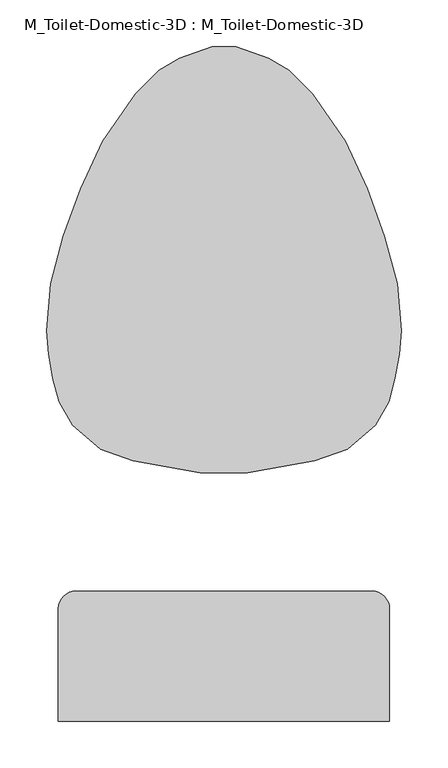
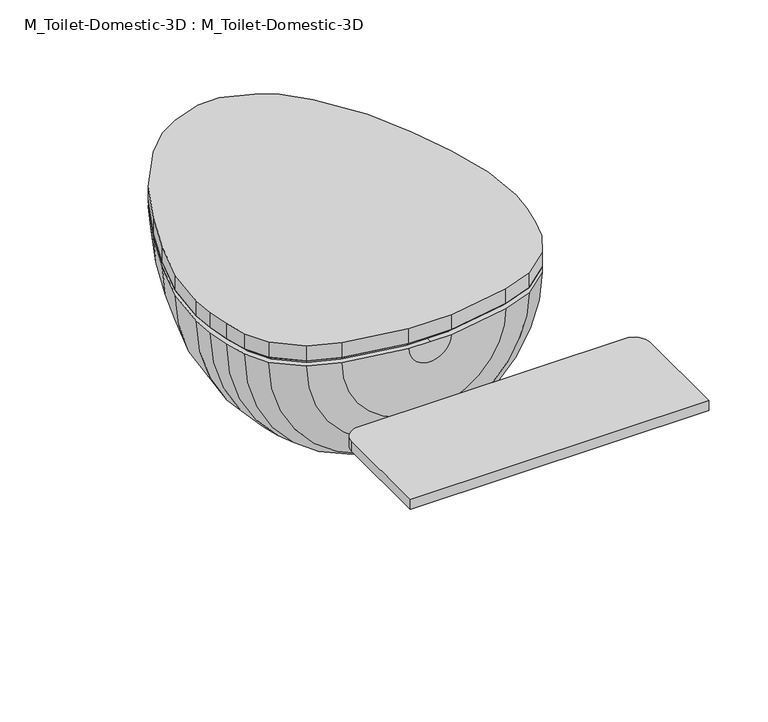
"""IFC4 building model written with IfcOpenShell, lengths in millimetres: flow terminal geometry, M_Toilet-Domestic-3D : M_Toilet-Domestic-3D."""

from ifc_helpers import new_model, si_unit, point, frame, frame_2d, origin, place, context, project, spatial, polyline, circle_curve, trimmed, segment, composite_curve, outline, extrude, faceted_brep, source, transform, mapped, element, save
from ifc_brep_helpers import plane_surface, revolved_surface, advanced_brep


def m_toilet_domestic_3d_m_toilet_domestic_3d_5530cc89(model_context):
    return source(origin(), model_context, "Body", "SolidModel", [
        advanced_brep(
        [(-25.4, -152.4, 361.95), (0.0, -152.4, 361.95), (0.0, -133.6394123, 361.95), (-22.0920022, -133.6394123, 361.95), (-94.1172813, -120.9394123, 361.95), (-121.9980886, -110.7916284, 361.95), (-146.1085923, -90.5605136, 361.95), (-159.5484355, -68.2281551, 361.95), (-165.101298, -47.5045901, 361.95), (-169.3087351, -23.6430284, 361.95), (-171.5645445, 2.1409906, 361.95), (-167.7238545, 46.0402777, 361.95), (-154.575847, 95.1093097, 361.95), (-136.654021, 144.3491221, 361.95), (-114.0255101, 192.8761202, 361.95), (-79.2146703, 243.0564036, 361.95), (-58.4178985, 263.8531754, 361.95), (-39.5113323, 274.7688865, 361.95), (-12.5224565, 284.592034, 361.95), (0.0, 284.592034, 361.95), (0.0, 304.8, 361.95), (-12.7, 304.8, 361.95), (-47.5929632, 292.1, 361.95), (-69.5900085, 279.4, 361.95), (-94.9900085, 254.0, 361.95), (-130.2307553, 203.2, 361.95), (-153.9191843, 152.4, 361.95), (-172.4088722, 101.6, 361.95), (-186.0724883, 50.6066907, 361.95), (-190.5, 0.0, 361.95), (-188.2862441, -25.3033453, 361.95), (-183.790496, -50.8, 361.95), (-176.9845865, -76.2, 361.95), (-162.5887836, -101.6, 361.95), (-132.3182423, -127.0, 361.95), (-97.4252791, -139.7, 361.95), (25.4, -152.4, 361.95), (97.4252791, -139.7, 361.95), (132.3182423, -127.0, 361.95), (162.5887836, -101.6, 361.95), (176.9845865, -76.2, 361.95), (183.790496, -50.8, 361.95), (188.2862441, -25.3033453, 361.95), (190.5, 0.0, 361.95), (186.0724883, 50.6066907, 361.95), (172.4088722, 101.6, 361.95), (153.9191843, 152.4, 361.95), (130.2307553, 203.2, 361.95), (94.9900085, 254.0, 361.95), (69.5900085, 279.4, 361.95), (47.5929632, 292.1, 361.95), (12.7, 304.8, 361.95), (12.5224565, 284.592034, 361.95), (39.5113323, 274.7688865, 361.95), (58.4178985, 263.8531754, 361.95), (79.2146703, 243.0564036, 361.95), (114.0255101, 192.8761202, 361.95), (136.654021, 144.3491221, 361.95), (154.575847, 95.1093097, 361.95), (167.7238545, 46.0402777, 361.95), (171.5645445, 2.1409906, 361.95), (169.3087351, -23.6430284, 361.95), (165.101298, -47.5045901, 361.95), (159.5484355, -68.2281551, 361.95), (146.1085923, -90.5605136, 361.95), (121.9980886, -110.7916284, 361.95), (94.1172813, -120.9394123, 361.95), (22.0920022, -133.6394123, 361.95)],
        [
            (0, 1),
            (1, 2),
            (2, 3),
            (3, 4),
            (4, 5),
            (5, 6),
            (6, 7),
            (7, 8),
            (8, 9),
            (9, 10),
            (10, 11),
            (11, 12),
            (12, 13),
            (13, 14),
            (14, 15),
            (15, 16),
            (16, 17),
            (17, 18),
            (18, 19),
            (19, 20),
            (20, 21),
            (21, 22),
            (22, 23),
            (23, 24),
            (24, 25),
            (25, 26),
            (26, 27),
            (27, 28),
            (28, 29),
            (29, 30),
            (30, 31),
            (31, 32),
            (32, 33),
            (33, 34),
            (34, 35),
            (35, 0),
            (36, 37),
            (37, 38),
            (38, 39),
            (39, 40),
            (40, 41),
            (41, 42),
            (42, 43),
            (43, 44),
            (44, 45),
            (45, 46),
            (46, 47),
            (47, 48),
            (48, 49),
            (49, 50),
            (50, 51),
            (51, 20),
            (19, 52),
            (52, 53),
            (53, 54),
            (54, 55),
            (55, 56),
            (56, 57),
            (57, 58),
            (58, 59),
            (59, 60),
            (60, 61),
            (61, 62),
            (62, 63),
            (63, 64),
            (64, 65),
            (65, 66),
            (66, 67),
            (67, 2),
            (1, 36),
            (36, 0, circle_curve(frame((0.0, -152.4, 361.95), z_axis=(0.0, 1.0, 0.0), x_axis=(-1.0, 0.0, 0.0)), 25.4)),
            (35, 37, circle_curve(frame((0.0, -139.7, 361.95), z_axis=(0.0, -1.0, 0.0), x_axis=(-1.0, 0.0, 0.0)), 97.4252791)),
            (34, 38, circle_curve(frame((0.0, -127.0, 361.95), z_axis=(0.0, -1.0, 0.0), x_axis=(-1.0, 0.0, 0.0)), 132.3182423)),
            (33, 39, circle_curve(frame((0.0, -101.6, 361.95), z_axis=(0.0, -1.0, 0.0), x_axis=(-1.0, 0.0, 0.0)), 162.5887836)),
            (32, 40, circle_curve(frame((0.0, -76.2, 361.95), z_axis=(0.0, -1.0, 0.0), x_axis=(-1.0, 0.0, 0.0)), 176.9845865)),
            (31, 41, circle_curve(frame((0.0, -50.8, 361.95), z_axis=(0.0, -1.0, 0.0), x_axis=(-1.0, 0.0, 0.0)), 183.790496)),
            (30, 42, circle_curve(frame((0.0, -25.3033453, 361.95), z_axis=(0.0, -1.0, 0.0), x_axis=(-1.0, 0.0, 0.0)), 188.2862441)),
            (29, 43, circle_curve(frame((0.0, 0.0, 361.95), z_axis=(0.0, -1.0, 0.0), x_axis=(-1.0, 0.0, 0.0)), 190.5)),
            (28, 44, circle_curve(frame((0.0, 50.6066907, 361.95), z_axis=(0.0, -1.0, 0.0), x_axis=(-1.0, 0.0, 0.0)), 186.0724883)),
            (27, 45, circle_curve(frame((0.0, 101.6, 361.95), z_axis=(0.0, -1.0, 0.0), x_axis=(-1.0, 0.0, 0.0)), 172.4088722)),
            (26, 46, circle_curve(frame((0.0, 152.4, 361.95), z_axis=(0.0, -1.0, 0.0), x_axis=(-1.0, 0.0, 0.0)), 153.9191843)),
            (25, 47, circle_curve(frame((0.0, 203.2, 361.95), z_axis=(0.0, -1.0, 0.0), x_axis=(-1.0, 0.0, 0.0)), 130.2307553)),
            (24, 48, circle_curve(frame((0.0, 254.0, 361.95), z_axis=(0.0, -1.0, 0.0), x_axis=(-1.0, 0.0, 0.0)), 94.9900085)),
            (23, 49, circle_curve(frame((0.0, 279.4, 361.95), z_axis=(0.0, -1.0, 0.0), x_axis=(-1.0, 0.0, 0.0)), 69.5900085)),
            (22, 50, circle_curve(frame((0.0, 292.1, 361.95), z_axis=(0.0, -1.0, 0.0), x_axis=(-1.0, 0.0, 0.0)), 47.5929632)),
            (21, 51, circle_curve(frame((0.0, 304.8, 361.95), z_axis=(0.0, -1.0, 0.0), x_axis=(-1.0, 0.0, 0.0)), 12.7)),
            (18, 52, circle_curve(frame((0.0, 284.592034, 361.95), z_axis=(0.0, -1.0, 0.0), x_axis=(-1.0, 0.0, 0.0)), 12.5224565)),
            (17, 53, circle_curve(frame((0.0, 274.7688865, 361.95), z_axis=(0.0, -1.0, 0.0), x_axis=(-1.0, 0.0, 0.0)), 39.5113323)),
            (16, 54, circle_curve(frame((0.0, 263.8531754, 361.95), z_axis=(0.0, -1.0, 0.0), x_axis=(-1.0, 0.0, 0.0)), 58.4178985)),
            (15, 55, circle_curve(frame((0.0, 243.0564036, 361.95), z_axis=(0.0, -1.0, 0.0), x_axis=(-1.0, 0.0, 0.0)), 79.2146703)),
            (14, 56, circle_curve(frame((0.0, 192.8761202, 361.95), z_axis=(0.0, -1.0, 0.0), x_axis=(-1.0, 0.0, 0.0)), 114.0255101)),
            (13, 57, circle_curve(frame((0.0, 144.3491221, 361.95), z_axis=(0.0, -1.0, 0.0), x_axis=(-1.0, 0.0, 0.0)), 136.654021)),
            (12, 58, circle_curve(frame((0.0, 95.1093097, 361.95), z_axis=(0.0, -1.0, 0.0), x_axis=(-1.0, 0.0, 0.0)), 154.575847)),
            (11, 59, circle_curve(frame((0.0, 46.0402777, 361.95), z_axis=(0.0, -1.0, 0.0), x_axis=(-1.0, 0.0, 0.0)), 167.7238545)),
            (10, 60, circle_curve(frame((0.0, 2.1409906, 361.95), z_axis=(0.0, -1.0, 0.0), x_axis=(-1.0, 0.0, 0.0)), 171.5645445)),
            (9, 61, circle_curve(frame((0.0, -23.6430284, 361.95), z_axis=(0.0, -1.0, 0.0), x_axis=(-1.0, 0.0, 0.0)), 169.3087351)),
            (8, 62, circle_curve(frame((0.0, -47.5045901, 361.95), z_axis=(0.0, -1.0, 0.0), x_axis=(-1.0, 0.0, 0.0)), 165.101298)),
            (7, 63, circle_curve(frame((0.0, -68.2281551, 361.95), z_axis=(0.0, -1.0, 0.0), x_axis=(-1.0, 0.0, 0.0)), 159.5484355)),
            (6, 64, circle_curve(frame((0.0, -90.5605136, 361.95), z_axis=(0.0, -1.0, 0.0), x_axis=(-1.0, 0.0, 0.0)), 146.1085923)),
            (5, 65, circle_curve(frame((0.0, -110.7916284, 361.95), z_axis=(0.0, -1.0, 0.0), x_axis=(-1.0, 0.0, 0.0)), 121.9980886)),
            (4, 66, circle_curve(frame((0.0, -120.9394123, 361.95), z_axis=(0.0, -1.0, 0.0), x_axis=(-1.0, 0.0, 0.0)), 94.1172813)),
            (3, 67, circle_curve(frame((0.0, -133.6394123, 361.95), z_axis=(0.0, -1.0, 0.0), x_axis=(-1.0, 0.0, 0.0)), 22.0920022)),
        ],
        [
            plane_surface(frame((0.0, -175.1599017, 361.95), z_axis=(0.0, 0.0, 1.0), x_axis=(-1.0, 0.0, 0.0))),
            plane_surface(frame((0.0, -175.1599017, 361.95), z_axis=(0.0, 0.0, 1.0), x_axis=(1.0, 0.0, 0.0))),
            revolved_surface(polyline([(-25.4, -152.4, 361.95), (-97.4252791, -139.7, 361.95)]), (0.0, -175.1599017, 361.95), (0.0, 1.0, 0.0)),
            revolved_surface(polyline([(-97.4252791, -139.7, 361.95), (-132.3182423, -127.0, 361.95)]), (0.0, -175.1599017, 361.95), (0.0, 1.0, 0.0)),
            revolved_surface(polyline([(-132.3182423, -127.0, 361.95), (-162.5887836, -101.6, 361.95)]), (0.0, -175.1599017, 361.95), (0.0, 1.0, 0.0)),
            revolved_surface(polyline([(-162.5887836, -101.6, 361.95), (-176.9845865, -76.2, 361.95)]), (0.0, -175.1599017, 361.95), (0.0, 1.0, 0.0)),
            revolved_surface(polyline([(-176.9845865, -76.2, 361.95), (-183.790496, -50.8, 361.95)]), (0.0, -175.1599017, 361.95), (0.0, 1.0, 0.0)),
            revolved_surface(polyline([(-183.790496, -50.8, 361.95), (-188.2862441, -25.3033453, 361.95)]), (0.0, -175.1599017, 361.95), (0.0, 1.0, 0.0)),
            revolved_surface(polyline([(-188.2862441, -25.3033453, 361.95), (-190.5, 0.0, 361.95)]), (0.0, -175.1599017, 361.95), (0.0, 1.0, 0.0)),
            revolved_surface(polyline([(-190.5, 0.0, 361.95), (-186.0724883, 50.6066907, 361.95)]), (0.0, -175.1599017, 361.95), (0.0, 1.0, 0.0)),
            revolved_surface(polyline([(-186.0724883, 50.6066907, 361.95), (-172.4088722, 101.6, 361.95)]), (0.0, -175.1599017, 361.95), (0.0, 1.0, 0.0)),
            revolved_surface(polyline([(-172.4088722, 101.6, 361.95), (-153.9191843, 152.4, 361.95)]), (0.0, -175.1599017, 361.95), (0.0, 1.0, 0.0)),
            revolved_surface(polyline([(-153.9191843, 152.4, 361.95), (-130.2307553, 203.2, 361.95)]), (0.0, -175.1599017, 361.95), (0.0, 1.0, 0.0)),
            revolved_surface(polyline([(-130.2307553, 203.2, 361.95), (-94.9900085, 254.0, 361.95)]), (0.0, -175.1599017, 361.95), (0.0, 1.0, 0.0)),
            revolved_surface(polyline([(-94.9900085, 254.0, 361.95), (-69.5900085, 279.4, 361.95)]), (0.0, -175.1599017, 361.95), (0.0, 1.0, 0.0)),
            revolved_surface(polyline([(-69.5900085, 279.4, 361.95), (-47.5929632, 292.1, 361.95)]), (0.0, -175.1599017, 361.95), (0.0, 1.0, 0.0)),
            revolved_surface(polyline([(-47.5929632, 292.1, 361.95), (-12.7, 304.8, 361.95)]), (0.0, -175.1599017, 361.95), (0.0, 1.0, 0.0)),
            plane_surface(frame((0.0, 304.8, 361.95), z_axis=(0.0, 1.0, 0.0), x_axis=(-1.0, 0.0, 0.0))),
            plane_surface(frame((0.0, 284.592034, 361.95), z_axis=(0.0, -1.0, 0.0), x_axis=(-1.0, 0.0, 0.0))),
            revolved_surface(polyline([(-12.5224565, 284.592034, 361.95), (-39.5113323, 274.7688865, 361.95)]), (0.0, -175.1599017, 361.95), (0.0, 1.0, 0.0)),
            revolved_surface(polyline([(-39.5113323, 274.7688865, 361.95), (-58.4178985, 263.8531754, 361.95)]), (0.0, -175.1599017, 361.95), (0.0, 1.0, 0.0)),
            revolved_surface(polyline([(-58.4178985, 263.8531754, 361.95), (-79.2146703, 243.0564036, 361.95)]), (0.0, -175.1599017, 361.95), (0.0, 1.0, 0.0)),
            revolved_surface(polyline([(-79.2146703, 243.0564036, 361.95), (-114.0255101, 192.8761202, 361.95)]), (0.0, -175.1599017, 361.95), (0.0, 1.0, 0.0)),
            revolved_surface(polyline([(-114.0255101, 192.8761202, 361.95), (-136.654021, 144.3491221, 361.95)]), (0.0, -175.1599017, 361.95), (0.0, 1.0, 0.0)),
            revolved_surface(polyline([(-136.654021, 144.3491221, 361.95), (-154.575847, 95.1093097, 361.95)]), (0.0, -175.1599017, 361.95), (0.0, 1.0, 0.0)),
            revolved_surface(polyline([(-154.575847, 95.1093097, 361.95), (-167.7238545, 46.0402777, 361.95)]), (0.0, -175.1599017, 361.95), (0.0, 1.0, 0.0)),
            revolved_surface(polyline([(-167.7238545, 46.0402777, 361.95), (-171.5645445, 2.1409906, 361.95)]), (0.0, -175.1599017, 361.95), (0.0, 1.0, 0.0)),
            revolved_surface(polyline([(-171.5645445, 2.1409906, 361.95), (-169.3087351, -23.6430284, 361.95)]), (0.0, -175.1599017, 361.95), (0.0, 1.0, 0.0)),
            revolved_surface(polyline([(-169.3087351, -23.6430284, 361.95), (-165.101298, -47.5045901, 361.95)]), (0.0, -175.1599017, 361.95), (0.0, 1.0, 0.0)),
            revolved_surface(polyline([(-165.101298, -47.5045901, 361.95), (-159.5484355, -68.2281551, 361.95)]), (0.0, -175.1599017, 361.95), (0.0, 1.0, 0.0)),
            revolved_surface(polyline([(-159.5484355, -68.2281551, 361.95), (-146.1085923, -90.5605136, 361.95)]), (0.0, -175.1599017, 361.95), (0.0, 1.0, 0.0)),
            revolved_surface(polyline([(-146.1085923, -90.5605136, 361.95), (-121.9980886, -110.7916284, 361.95)]), (0.0, -175.1599017, 361.95), (0.0, 1.0, 0.0)),
            revolved_surface(polyline([(-121.9980886, -110.7916284, 361.95), (-94.1172813, -120.9394123, 361.95)]), (0.0, -175.1599017, 361.95), (0.0, 1.0, 0.0)),
            revolved_surface(polyline([(-94.1172813, -120.9394123, 361.95), (-22.0920022, -133.6394123, 361.95)]), (0.0, -175.1599017, 361.95), (0.0, 1.0, 0.0)),
            plane_surface(frame((0.0, -133.6394123, 361.95), z_axis=(0.0, 1.0, 0.0), x_axis=(-1.0, 0.0, 0.0))),
            plane_surface(frame((0.0, -152.4, 361.95), z_axis=(0.0, -1.0, 0.0), x_axis=(-1.0, 0.0, 0.0))),
        ],
        [
            (0, [[1, 2, 3, 4, 5, 6, 7, 8, 9, 10, 11, 12, 13, 14, 15, 16, 17, 18, 19, 20, 21, 22, 23, 24, 25, 26, 27, 28, 29, 30, 31, 32, 33, 34, 35, 36]]),
            (1, [[37, 38, 39, 40, 41, 42, 43, 44, 45, 46, 47, 48, 49, 50, 51, 52, -20, 53, 54, 55, 56, 57, 58, 59, 60, 61, 62, 63, 64, 65, 66, 67, 68, 69, -2, 70]]),
            (2, [[-37, 71, -36, 72]]),
            (3, [[-38, -72, -35, 73]]),
            (4, [[-39, -73, -34, 74]]),
            (5, [[-40, -74, -33, 75]]),
            (6, [[-41, -75, -32, 76]]),
            (7, [[-42, -76, -31, 77]]),
            (8, [[-43, -77, -30, 78]]),
            (9, [[-44, -78, -29, 79]]),
            (10, [[-45, -79, -28, 80]]),
            (11, [[-46, -80, -27, 81]]),
            (12, [[-47, -81, -26, 82]]),
            (13, [[-48, -82, -25, 83]]),
            (14, [[-49, -83, -24, 84]]),
            (15, [[-50, -84, -23, 85]]),
            (16, [[-51, -85, -22, 86]]),
            (17, [[-52, -86, -21]]),
            (18, [[-53, -19, 87]]),
            (19, [[-54, -87, -18, 88]]),
            (20, [[-55, -88, -17, 89]]),
            (21, [[-56, -89, -16, 90]]),
            (22, [[-57, -90, -15, 91]]),
            (23, [[-58, -91, -14, 92]]),
            (24, [[-59, -92, -13, 93]]),
            (25, [[-60, -93, -12, 94]]),
            (26, [[-61, -94, -11, 95]]),
            (27, [[-62, -95, -10, 96]]),
            (28, [[-63, -96, -9, 97]]),
            (29, [[-64, -97, -8, 98]]),
            (30, [[-65, -98, -7, 99]]),
            (31, [[-66, -99, -6, 100]]),
            (32, [[-67, -100, -5, 101]]),
            (33, [[-68, -101, -4, 102]]),
            (34, [[-69, -102, -3]]),
            (35, [[-70, -1, -71]]),
        ],
    ),
        faceted_brep([(-97.4252791, -139.7, 368.3), (-25.4, -152.4, 368.3), (25.4, -152.4, 368.3), (97.4252791, -139.7, 368.3), (132.3182423, -127.0, 368.3), (162.5887836, -101.6, 368.3), (176.9845865, -76.2, 368.3), (183.790496, -50.8, 368.3), (188.2862441, -25.3033453, 368.3), (190.5, 0.0, 368.3), (186.0724883, 50.6066907, 368.3), (172.4088722, 101.6, 368.3), (153.9191843, 152.4, 368.3), (130.2307553, 203.2, 368.3), (94.9900085, 254.0, 368.3), (69.5900085, 279.4, 368.3), (47.5929632, 292.1, 368.3), (12.7, 304.8, 368.3), (-12.7, 304.8, 368.3), (-47.5929632, 292.1, 368.3), (-69.5900085, 279.4, 368.3), (-94.9900085, 254.0, 368.3), (-130.2307553, 203.2, 368.3), (-153.9191843, 152.4, 368.3), (-172.4088722, 101.6, 368.3), (-186.0724883, 50.6066907, 368.3), (-190.5, 0.0, 368.3), (-188.2862441, -25.3033453, 368.3), (-183.790496, -50.8, 368.3), (-176.9845865, -76.2, 368.3), (-162.5887836, -101.6, 368.3), (-132.3182423, -127.0, 368.3), (-95.7755003, -133.5429415, 361.95), (-129.0942628, -121.4159037, 361.95), (-157.6293435, -97.472128, 361.95), (-171.060664, -73.773864, 361.95), (-177.5851102, -49.4242991, 361.95), (-181.9845715, -24.4737144, 361.95), (-184.125744, 0.0, 361.95), (-179.7950716, 49.4998127, 361.95), (-166.347, 99.688699, 361.95), (-148.0469602, 149.9676451, 361.95), (-124.7045808, 200.0255393, 361.95), (-90.0971582, 249.9125941, 361.95), (-65.691017, 274.3187354, 361.95), (-44.8990862, 286.3229622, 361.95), (-11.5803237, 298.45, 361.95), (11.5803237, 298.45, 361.95), (44.8990862, 286.3229622, 361.95), (65.691017, 274.3187354, 361.95), (90.0971582, 249.9125941, 361.95), (124.7045808, 200.0255393, 361.95), (148.0469602, 149.9676451, 361.95), (166.347, 99.688699, 361.95), (179.7950716, 49.4998127, 361.95), (184.125744, 0.0, 361.95), (181.9845715, -24.4737144, 361.95), (177.5851102, -49.4242991, 361.95), (171.060664, -73.773864, 361.95), (157.6293435, -97.472128, 361.95), (129.0942628, -121.4159037, 361.95), (95.7755003, -133.5429415, 361.95), (24.844447, -146.05, 361.95), (-24.844447, -146.05, 361.95)], [[[0, 1, 2, 3, 4, 5, 6, 7, 8, 9, 10, 11, 12, 13, 14, 15, 16, 17, 18, 19, 20, 21, 22, 23, 24, 25, 26, 27, 28, 29, 30, 31]], [[32, 33, 34, 35, 36, 37, 38, 39, 40, 41, 42, 43, 44, 45, 46, 47, 48, 49, 50, 51, 52, 53, 54, 55, 56, 57, 58, 59, 60, 61, 62, 63]], [[32, 0, 31, 33]], [[33, 31, 30, 34]], [[34, 30, 29, 35]], [[35, 29, 28, 36]], [[36, 28, 27, 37]], [[37, 27, 26, 38]], [[38, 26, 25, 39]], [[39, 25, 24, 40]], [[40, 24, 23, 41]], [[41, 23, 22, 42]], [[42, 22, 21, 43]], [[43, 21, 20, 44]], [[44, 20, 19, 45]], [[45, 19, 18, 46]], [[46, 18, 17, 47]], [[47, 17, 16, 48]], [[48, 16, 15, 49]], [[49, 15, 14, 50]], [[50, 14, 13, 51]], [[51, 13, 12, 52]], [[52, 12, 11, 53]], [[53, 11, 10, 54]], [[54, 10, 9, 55]], [[55, 9, 8, 56]], [[56, 8, 7, 57]], [[57, 7, 6, 58]], [[58, 6, 5, 59]], [[59, 5, 4, 60]], [[60, 4, 3, 61]], [[61, 3, 2, 62]], [[62, 2, 1, 63]], [[63, 1, 0, 32]]]),
        extrude(outline(composite_curve([segment(polyline([(177.8, -419.1), (-177.8, -419.1), (-177.8, -298.45)]), True, "CONTINUOUS"), segment(trimmed(circle_curve(frame_2d((-158.75, -298.45)), 19.05), [point((-177.8, -298.45))], [point((-158.75, -279.4))], False, "CARTESIAN"), True, "CONTINUOUS"), segment(polyline([(-158.75, -279.4), (158.75, -279.4)]), True, "CONTINUOUS"), segment(trimmed(circle_curve(frame_2d((158.75, -298.45)), 19.05), [point((158.75, -279.4))], [point((177.8, -298.45))], False, "CARTESIAN"), True, "CONTINUOUS"), segment(polyline([(177.8, -298.45), (177.8, -419.1)]), True, "CONTINUOUS")], self_intersect=False)), frame((0.0, 0.0, 374.65), z_axis=(0.0, 0.0, 1.0), x_axis=(1.0, 0.0, 0.0)), (0.0, 0.0, 1.0), 12.5681453),
        extrude(outline(polyline([(-162.5887836, -101.6), (-176.9845865, -76.2), (-183.790496, -50.8), (-188.2862441, -25.3033453), (-190.5, 0.0), (-186.0724883, 50.6066907), (-172.4088722, 101.6), (-153.9191843, 152.4), (-130.2307553, 203.2), (-94.9900085, 254.0), (-69.5900085, 279.4), (-47.5929632, 292.1), (-12.7, 304.8), (12.7, 304.8), (47.5929632, 292.1), (69.5900085, 279.4), (94.9900085, 254.0), (130.2307553, 203.2), (153.9191843, 152.4), (172.4088722, 101.6), (186.0724883, 50.6066907), (190.5, 0.0), (188.2862441, -25.3033453), (183.790496, -50.8), (176.9845865, -76.2), (162.5887836, -101.6), (132.3182423, -127.0), (97.4252791, -139.7), (25.4, -152.4), (-25.4, -152.4), (-97.4252791, -139.7), (-132.3182423, -127.0), (-162.5887836, -101.6)])), frame((0.0, 0.0, 368.3), z_axis=(0.0, 0.0, 1.0), x_axis=(1.0, 0.0, 0.0)), (0.0, 0.0, 1.0), 19.05),
    ])


if __name__ == "__main__":
    model = new_model("IFC4")
    model_context = context("Model", 3, world=origin())
    ifc_project = project(units=[si_unit("LENGTHUNIT", "METRE", prefix="MILLI")], contexts=[model_context])
    site = spatial("IfcSite", under=ifc_project)
    building = spatial("IfcBuilding", under=site)
    placement = place(None, origin())
    m_toilet_domestic_3d_m_toilet_domestic_3d_shape = m_toilet_domestic_3d_m_toilet_domestic_3d_5530cc89(model_context)
    element("IfcFlowTerminal", 1, ObjectType="M_Toilet-Domestic-3D : M_Toilet-Domestic-3D", at=placement, inside=building, context=model_context, shape_type="MappedRepresentation", body=[
        mapped(m_toilet_domestic_3d_m_toilet_domestic_3d_shape, transform((0.0, 0.0, 0.0), x_axis=(1.0, 0.0, 0.0), y_axis=(0.0, 1.0, 0.0), z_axis=(0.0, 0.0, 1.0))),
    ])
    save(model, "model.ifc")

# Revit data of these elements
# Type "M_Toilet-Domestic-3D : M_Toilet-Domestic-3D"
#   Bowl/Basin Material = Porcelain, Linen
#   Seat Material = Laminate, Linen, Matte
#   Default Elevation = 0
# Element 1 (IfcFlowTerminal, "M_Toilet-Domestic-3D : M_Toilet-Domestic-3D")
#   Materials on its faces: "Porcelain, Linen", "Laminate, Linen, Matte"
# Materials
#   "Porcelain, Linen": class "Ceramic", colour RGB 249 239 230, transparency 0, Description = "Porcelain, linen", Cost = 0
#   "Laminate, Linen, Matte": class "Plastic", colour RGB 249 239 230, transparency 0, Description = "Plastic Laminate - Linen, Matte", Cost = 0
